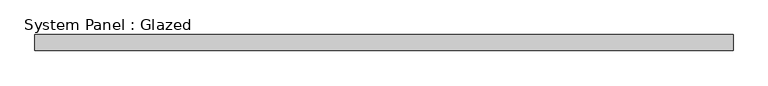
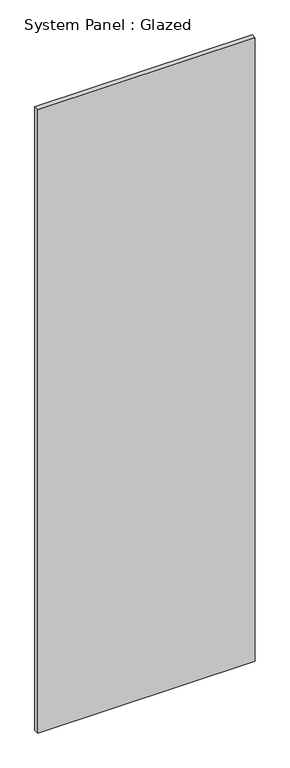
"""IFC4 building model written with IfcOpenShell, lengths in millimetres: plate geometry, System Panel : Glazed."""

from ifc_helpers import new_model, si_unit, origin, origin_with_axes, place, context, project, spatial, polyline, outline, extrude, source, transform, mapped, element, save


def system_panel_glazed_3d2c66d7(model_context):
    return source(origin(), model_context, "Body", "SweptSolid", [
        extrude(outline(polyline([(558.25, 19.05), (-558.25, 19.05), (-558.25, 44.45), (558.25, 44.45), (558.25, 19.05)])), origin_with_axes(), (0.0, 0.0, 1.0), 3379.9820397),
    ])


if __name__ == "__main__":
    model = new_model("IFC4")
    model_context = context("Model", 3, world=origin())
    ifc_project = project(units=[si_unit("LENGTHUNIT", "METRE", prefix="MILLI")], contexts=[model_context])
    site = spatial("IfcSite", under=ifc_project)
    building = spatial("IfcBuilding", under=site)
    placement = place(None, origin())
    system_panel_glazed_shape = system_panel_glazed_3d2c66d7(model_context)
    element("IfcPlate", 1, ObjectType="System Panel : Glazed", at=placement, inside=building, context=model_context, shape_type="MappedRepresentation", body=[
        mapped(system_panel_glazed_shape, transform((0.0, 0.0, 0.0), x_axis=(1.0, 0.0, 0.0), y_axis=(0.0, 1.0, 0.0), z_axis=(0.0, 0.0, 1.0))),
    ])
    save(model, "model.ifc")

# Revit data of these elements
# Type "System Panel : Glazed"
#   Construction Type Id = "GSP4R"
#   Analytic Construction = "1/8 in Pilkington single glazing"
#   Visual Light Transmittance = 0.9
#   Solar Heat Gain Coefficient = 0.86
#   Heat Transfer Coefficient (U) = 1.18115 BTU/(h·ft²·°F)
#   Define Thermal Properties by = 1
# Element 1 (IfcPlate, "System Panel : Glazed")
#   Materials on its faces: "Glass"
# Materials
#   "Glass": class "Glass", colour RGB 0 128 192, transparency 0.75, Description = "Soda Lime Glass", Cost = 0
